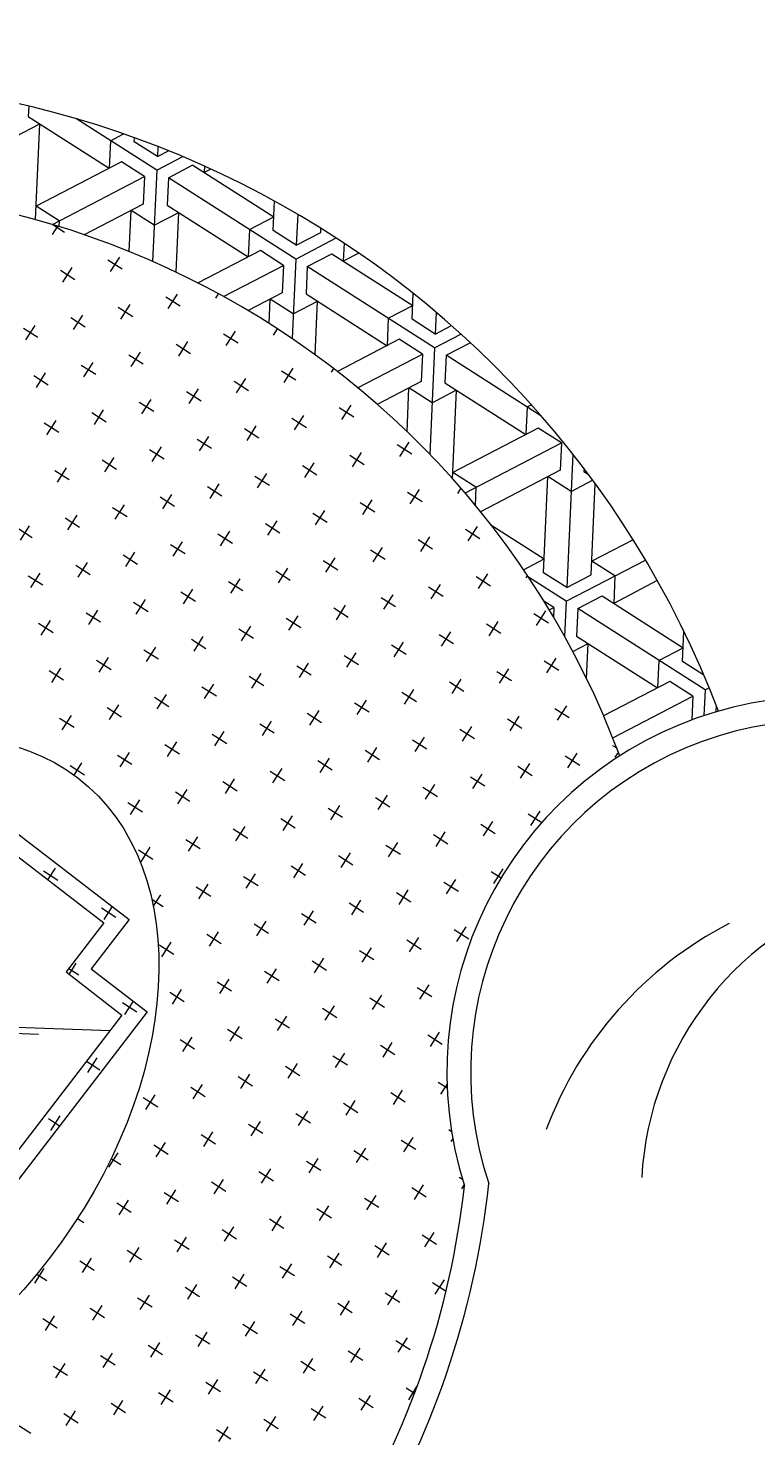
# Model space of a CAD drawing. Units: inches. Extents: x -4843 to -3402, y -164 to 3629.
# Tile 13 of 22: x -4487 to -4467, y 864 to 902. Entities that reach past the tile are written whole.
import ezdxf

# ---------------------------------------------------------------- set-up
doc = ezdxf.new("R2010")
doc.units = ezdxf.units.IN
doc.layers.add('A-ANNO-DIMS', color=2, linetype='Continuous', lineweight=18)
doc.layers.add('furniture', color=6, linetype='Continuous', lineweight=18)
doc.styles.get("Standard").update_dxf_attribs({"font": 'arial.ttf'})
doc.dimstyles.get("Standard").update_dxf_attribs({"dimtxt": 0.18, "dimasz": 0.18, "dimexe": 0.18, "dimexo": 0.0625, "dimgap": 0.09, "dimtad": 0, "dimtih": 1, "dimtoh": 1, "dimdec": 4, "dimzin": 0, "dimdsep": 46, "dimtxsty": 'Standard', "dimcen": 0.09, "dimadec": 0, "dimazin": 0, "dimtfac": 1, "dimtdec": 4, "dimtofl": 0, "dimtmove": 0, "dimatfit": 3, "dimfxl": 1, "dimtolj": 1, "dimtzin": 0, "dimarcsym": 0})

# ---------------------------------------------------------------- blocks, each defined once
blk = doc.blocks.new('A$C30AE1D3B')
for p, q in [((999.1, 1767.5, -685.7), (983.6, 1760.2, -685.7)), ((994.5, 1754.8, -685.7), (989.7, 1764.9, -685.7)), ((1049.7, 1749, -685.7), (1032.4, 1741, -685.7)), ((1045.1, 1736.4, -685.7), (1037, 1753.6, -685.7)), ((1095.7, 1717.9, -685.7), (1087.7, 1735.2, -685.7)), ((976, 1704.2, -685.7), (968, 1721.4, -685.7)), ((1100.3, 1730.6, -685.7), (1083.1, 1722.6, -685.7)), ((980.6, 1716.8, -685.7), (963.4, 1708.8, -685.7)), ((1026.7, 1685.7, -685.7), (1018.6, 1703, -685.7)), ((1151, 1712.2, -685.7), (1133.7, 1704.1, -685.7)), ((1146.3, 1699.5, -685.7), (1138.3, 1716.8, -685.7)), ((907, 1672, -685.7), (899.5, 1688, -685.7)), ((1031.3, 1698.4, -685.7), (1014, 1690.4, -685.7)), ((1201.6, 1693.7, -685.7), (1184.3, 1685.7, -685.7)), ((1197, 1681.1, -685.7), (1188.9, 1698.4, -685.7)), ((911.6, 1684.6, -685.7), (894.3, 1676.6, -685.7)), ((957.6, 1653.5, -685.7), (949.5, 1670.8, -685.7)), ((1081.9, 1680, -685.7), (1064.6, 1671.9, -685.7)), ((1077.3, 1667.3, -685.7), (1069.2, 1684.6, -685.7)), ((962.2, 1666.2, -685.7), (944.9, 1658.1, -685.7)), ((1132.5, 1661.5, -685.7), (1115.3, 1653.5, -685.7)), ((1127.9, 1648.9, -685.7), (1119.9, 1666.2, -685.7)), ((1012.8, 1647.8, -685.7), (995.6, 1639.7, -685.7)), ((1008.2, 1635.1, -685.7), (1000.2, 1652.4, -685.7)), ((1183.2, 1643.1, -685.7), (1165.9, 1635.1, -685.7)), ((1178.6, 1630.5, -685.7), (1170.5, 1647.7, -685.7)), ((893.1, 1634, -685.7), (875.9, 1625.9, -685.7)), ((888.5, 1621.3, -685.7), (880.5, 1638.6, -685.7)), ((1063.5, 1629.3, -685.7), (1046.2, 1621.3, -685.7)), ((1058.9, 1616.7, -685.7), (1050.8, 1633.9, -685.7)), ((1233.8, 1624.7, -685.7), (1216.5, 1616.6, -685.7)), ((1229.2, 1612, -685.7), (1221.1, 1629.3, -685.7)), ((943.8, 1615.6, -685.7), (926.5, 1607.5, -685.7)), ((939.2, 1602.9, -685.7), (931.1, 1620.2, -685.7)), ((1114.1, 1610.9, -685.7), (1096.8, 1602.9, -685.7)), ((1109.5, 1598.3, -685.7), (1101.4, 1615.5, -685.7)), ((1279.8, 1593.6, -685.7), (1271.8, 1610.9, -685.7)), ((819.5, 1589.1, -685.7), (817.6, 1593.1, -685.7)), ((824.1, 1601.8, -685.7), (819.4, 1599.6, -685.7)), ((994.4, 1597.1, -685.7), (977.1, 1589.1, -685.7)), ((989.8, 1584.5, -685.7), (981.7, 1601.7, -685.7)), ((1160.1, 1579.8, -685.7), (1152.1, 1597.1, -685.7)), ((1284.4, 1606.3, -685.7), (1267.2, 1598.2, -685.7)), ((874.7, 1583.4, -685.7), (857.4, 1575.3, -685.7)), ((870.1, 1570.7, -685.7), (862.1, 1588, -685.7)), ((1045, 1578.7, -685.7), (1027.8, 1570.7, -685.7)), ((1040.4, 1566.1, -685.7), (1032.4, 1583.3, -685.7)), ((1164.7, 1592.5, -685.7), (1147.5, 1584.4, -685.7)), ((1210.8, 1561.4, -685.7), (1202.7, 1578.7, -685.7)), ((1335.1, 1587.8, -685.7), (1317.8, 1579.8, -685.7)), ((1330.4, 1575.2, -685.7), (1322.4, 1592.4, -685.7)), ((925.3, 1564.9, -685.7), (908.1, 1556.9, -685.7)), ((920.7, 1552.3, -685.7), (912.7, 1569.5, -685.7)), ((1091.1, 1547.6, -685.7), (1083, 1564.9, -685.7)), ((1215.4, 1574.1, -685.7), (1198.1, 1566, -685.7)), ((1381.1, 1556.7, -685.7), (1373, 1574, -685.7)), ((805.7, 1551.2, -685.7), (802.7, 1549.8, -685.7)), ((976, 1546.5, -685.7), (958.7, 1538.5, -685.7)), ((971.4, 1533.8, -685.7), (963.3, 1551.1, -685.7)), ((1095.7, 1560.3, -685.7), (1078.4, 1552.2, -685.7)), ((1141.7, 1529.2, -685.7), (1133.6, 1546.5, -685.7)), ((1266, 1555.6, -685.7), (1248.7, 1547.6, -685.7)), ((1261.4, 1543, -685.7), (1253.3, 1560.2, -685.7)), ((801, 1538.5, -685.7), (799.4, 1542, -685.7)), ((856.3, 1532.7, -685.7), (839, 1524.7, -685.7)), ((851.7, 1520.1, -685.7), (843.6, 1537.3, -685.7)), ((1022, 1515.4, -685.7), (1014, 1532.7, -685.7)), ((1146.3, 1541.9, -685.7), (1129, 1533.8, -685.7)), ((1316.6, 1537.2, -685.7), (1299.4, 1529.1, -685.7)), ((1312, 1524.5, -685.7), (1304, 1541.8, -685.7)), ((902.3, 1501.6, -685.7), (894.3, 1518.9, -685.7)), ((1026.6, 1528.1, -685.7), (1009.3, 1520, -685.7)), ((1196.9, 1523.4, -685.7), (1179.7, 1515.4, -685.7)), ((1192.3, 1510.8, -685.7), (1184.3, 1528, -685.7)), ((787.2, 1500.5, -685.7), (775.6, 1495.1, -685.7)), ((906.9, 1514.3, -685.7), (889.7, 1506.3, -685.7)), ((952.9, 1483.2, -685.7), (944.9, 1500.5, -685.7)), ((1077.2, 1509.6, -685.7), (1060, 1501.6, -685.7)), ((1072.6, 1497, -685.7), (1064.6, 1514.3, -685.7)), ((1247.6, 1505, -685.7), (1230.3, 1496.9, -685.7)), ((1243, 1492.3, -685.7), (1234.9, 1509.6, -685.7)), ((782.6, 1487.9, -685.7), (777.6, 1498.6, -685.7)), ((833.2, 1469.4, -685.7), (825.2, 1486.7, -685.7)), ((957.5, 1495.9, -685.7), (940.3, 1487.8, -685.7)), ((1127.9, 1491.2, -685.7), (1110.6, 1483.2, -685.7)), ((1123.3, 1478.6, -685.7), (1115.2, 1495.8, -685.7)), ((1298.2, 1486.6, -685.7), (1280.9, 1478.5, -685.7)), ((1293.6, 1473.9, -685.7), (1285.5, 1491.2, -685.7)), ((837.9, 1482.1, -685.7), (820.6, 1474, -685.7)), ((883.9, 1451, -685.7), (875.8, 1468.3, -685.7)), ((1008.2, 1477.4, -685.7), (990.9, 1469.4, -685.7)), ((1003.6, 1464.8, -685.7), (995.5, 1482.1, -685.7)), ((1178.5, 1472.8, -685.7), (1161.2, 1464.7, -685.7)), ((1173.9, 1460.1, -685.7), (1165.8, 1477.4, -685.7)), ((764.2, 1437.2, -685.7), (756.1, 1454.5, -685.7)), ((888.5, 1463.7, -685.7), (871.2, 1455.6, -685.7)), ((1058.8, 1459, -685.7), (1041.5, 1451, -685.7)), ((1054.2, 1446.4, -685.7), (1046.2, 1463.6, -685.7)), ((1229.1, 1454.4, -685.7), (1211.9, 1446.3, -685.7)), ((1224.5, 1441.7, -685.7), (1216.5, 1459, -685.7)), ((768.8, 1449.9, -685.7), (751.5, 1441.8, -685.7)), ((939.1, 1445.2, -685.7), (921.9, 1437.2, -685.7)), ((934.5, 1432.6, -685.7), (926.5, 1449.9, -685.7)), ((1013.2, 1248.8, -685.7), (1537, 1439.4, -685.7)), ((1109.4, 1440.6, -685.7), (1092.2, 1432.5, -685.7)), ((1104.8, 1427.9, -685.7), (1096.8, 1445.2, -685.7)), ((1272.7, 1428.6, -685.7), (1267.1, 1440.5, -685.7)), ((819.4, 1431.5, -685.7), (802.2, 1423.4, -685.7)), ((814.8, 1418.8, -685.7), (806.8, 1436.1, -685.7)), ((989.8, 1426.8, -685.7), (972.5, 1418.8, -685.7)), ((985.1, 1414.2, -685.7), (977.1, 1431.4, -685.7)), ((1160.1, 1422.2, -685.7), (1142.8, 1414.1, -685.7)), ((1155.5, 1409.5, -685.7), (1147.4, 1426.8, -685.7)), ((1279.8, 1435.9, -685.7), (1262.5, 1427.9, -685.7)), ((870.1, 1413, -685.7), (852.8, 1405, -685.7)), ((865.5, 1400.4, -685.7), (857.4, 1417.6, -685.7)), ((1040.4, 1408.4, -685.7), (1023.1, 1400.3, -685.7)), ((1035.8, 1395.7, -685.7), (1027.7, 1413, -685.7)), ((1038.9, 1236.8, -685.7), (1525.1, 1413.8, -685.7)), ((1201.6, 1400.8, -685.7), (1198.1, 1408.3, -685.7)), ((750.4, 1399.3, -685.7), (733.1, 1391.2, -685.7)), ((745.8, 1386.6, -685.7), (737.7, 1403.9, -685.7)), ((920.7, 1394.6, -685.7), (903.4, 1386.6, -685.7)), ((916.1, 1382, -685.7), (908, 1399.2, -685.7)), ((1091, 1390, -685.7), (1073.8, 1381.9, -685.7)), ((1086.4, 1377.3, -685.7), (1078.4, 1394.6, -685.7)), ((801, 1380.8, -685.7), (783.7, 1372.8, -685.7)), ((796.4, 1368.2, -685.7), (788.3, 1385.4, -685.7)), ((971.3, 1376.2, -685.7), (954.1, 1368.1, -685.7)), ((966.7, 1363.5, -685.7), (958.7, 1380.8, -685.7)), ((1134.3, 1364.7, -685.7), (1129, 1376.1, -685.7)), ((681.3, 1367.1, -685.7), (664, 1359, -685.7)), ((676.7, 1354.4, -685.7), (668.6, 1371.7, -685.7)), ((851.6, 1362.4, -685.7), (834.4, 1354.4, -685.7)), ((847, 1349.7, -685.7), (839, 1367, -685.7)), ((1017.3, 1345.1, -685.7), (1009.3, 1362.4, -685.7)), ((1141.6, 1371.5, -685.7), (1124.4, 1363.5, -685.7)), ((731.9, 1348.6, -685.7), (714.7, 1340.6, -685.7)), ((727.3, 1336, -685.7), (719.3, 1353.2, -685.7)), ((902.3, 1344, -685.7), (885, 1335.9, -685.7)), ((897.7, 1331.3, -685.7), (889.6, 1348.6, -685.7)), ((1022, 1357.8, -685.7), (1004.7, 1349.7, -685.7)), ((1068, 1326.7, -685.7), (1059.9, 1343.9, -685.7)), ((612.2, 1334.9, -685.7), (595, 1326.8, -685.7)), ((607.6, 1322.2, -685.7), (602.2, 1333.9, -685.7)), ((782.6, 1330.2, -685.7), (765.3, 1322.2, -685.7)), ((778, 1317.5, -685.7), (769.9, 1334.8, -685.7)), ((948.3, 1312.9, -685.7), (940.2, 1330.2, -685.7)), ((1072.6, 1339.3, -685.7), (1055.3, 1331.3, -685.7)), ((662.9, 1316.4, -685.7), (645.6, 1308.4, -685.7)), ((658.3, 1303.8, -685.7), (650.2, 1321, -685.7)), ((833.2, 1311.8, -685.7), (815.9, 1303.7, -685.7)), ((828.6, 1299.1, -685.7), (820.5, 1316.4, -685.7)), ((952.9, 1325.6, -685.7), (935.6, 1317.5, -685.7)), ((998.9, 1294.5, -685.7), (990.9, 1311.7, -685.7)), ((298.1, 1300.5, -685.7), (302.2, 1306.3, -685.7)), ((299.5, 1279.4, -685.7), (315.8, 1302.7, -685.7)), ((314.6, 1278, -685.7), (329.7, 1299.5, -685.7)), ((543.2, 1302.7, -685.7), (525.9, 1294.6, -685.7)), ((538.6, 1290, -685.7), (531, 1306.3, -685.7)), ((713.5, 1298, -685.7), (696.2, 1289.9, -685.7)), ((708.9, 1285.3, -685.7), (700.9, 1302.6, -685.7)), ((879.2, 1280.7, -685.7), (871.2, 1298, -685.7)), ((1003.5, 1307.1, -685.7), (986.3, 1299.1, -685.7)), ((1173.9, 1302.5, -685.7), (1156.6, 1294.4, -685.7)), ((1169.2, 1289.8, -685.7), (1163, 1303.3, -685.7)), ((418.9, 1276.2, -685.7), (416.6, 1281.1, -685.7)), ((423.5, 1288.9, -685.7), (417.7, 1286.2, -685.7)), ((593.8, 1284.2, -685.7), (576.6, 1276.2, -685.7)), ((589.2, 1271.6, -685.7), (581.2, 1288.8, -685.7)), ((759.5, 1266.9, -685.7), (751.5, 1284.2, -685.7)), ((883.8, 1293.3, -685.7), (866.6, 1285.3, -685.7)), ((1041.5, 1293.2, -685.7), (1041.5, 1293.3, -685.7)), ((299.4, 1279.4, -685.7), (294.3, 1279.8, -685.7)), ((299.4, 1279.4, -685.7), (370.3, 1127.4, -685.7)), ((314.6, 1278, -685.7), (327.5, 1250.4, -685.7)), ((414.3, 1269.3, -685.7), (314.6, 1278, -685.7)), ((474.1, 1270.5, -685.7), (456.9, 1262.4, -685.7)), ((469.5, 1257.8, -685.7), (461.5, 1275.1, -685.7)), ((644.4, 1265.8, -685.7), (627.2, 1257.7, -685.7)), ((639.8, 1253.1, -685.7), (631.8, 1270.4, -685.7)), ((764.1, 1279.6, -685.7), (746.9, 1271.5, -685.7)), ((810.2, 1248.5, -685.7), (802.1, 1265.8, -685.7)), ((934.5, 1274.9, -685.7), (917.2, 1266.9, -685.7)), ((929.9, 1262.3, -685.7), (921.8, 1279.5, -685.7)), ((1104.8, 1270.3, -685.7), (1087.5, 1262.2, -685.7)), ((1099.6, 1258.9, -685.7), (1092.1, 1274.9, -685.7)), ((291.7, 1264.8, -685.7), (303.6, 1239.3, -685.7)), ((327.5, 1250.4, -685.7), (409.8, 1243.2, -685.7)), ((524.8, 1252, -685.7), (507.5, 1244, -685.7)), ((520.1, 1239.4, -685.7), (512.1, 1256.6, -685.7)), ((690.5, 1234.7, -685.7), (682.4, 1252, -685.7)), ((814.8, 1261.1, -685.7), (797.5, 1253.1, -685.7)), ((985.1, 1256.5, -685.7), (967.8, 1248.4, -685.7)), ((980.5, 1243.8, -685.7), (972.4, 1261.1, -685.7)), ((303.6, 1239.3, -685.7), (284.4, 1211.8, -685.7)), ((325.2, 1224.1, -685.7), (342.7, 1249.1, -685.7)), ((387.8, 1152.4, -685.7), (342.7, 1249.1, -685.7)), ((575.4, 1233.6, -685.7), (558.1, 1225.5, -685.7)), ((570.8, 1220.9, -685.7), (562.7, 1238.2, -685.7)), ((695.1, 1247.4, -685.7), (677.8, 1239.3, -685.7)), ((865.4, 1242.7, -685.7), (848.1, 1234.7, -685.7)), ((860.8, 1230.1, -685.7), (852.7, 1247.3, -685.7)), ((1040, 1175.2, -685.7), (1013.2, 1248.8, -685.7)), ((1035.7, 1238.1, -685.7), (1019.8, 1230.6, -685.7)), ((1031.1, 1225.4, -685.7), (1023.1, 1242.7, -685.7)), ((1065.6, 1163.2, -685.7), (1038.9, 1236.8, -685.7)), ((1381.8, 1022.6, -685.7), (1059.1, 1244.3, -685.7)), ((339.9, 1130.1, -685.7), (294.8, 1226.8, -685.7)), ((325.2, 1224.1, -685.7), (294.8, 1226.8, -685.7)), ((455.7, 1219.8, -685.7), (438.4, 1211.8, -685.7)), ((451.1, 1207.2, -685.7), (443, 1224.4, -685.7)), ((621.4, 1202.5, -685.7), (613.4, 1219.8, -685.7)), ((745.7, 1228.9, -685.7), (728.4, 1220.9, -685.7)), ((741.1, 1216.3, -685.7), (733.1, 1233.5, -685.7)), ((916, 1224.3, -685.7), (898.8, 1216.2, -685.7)), ((911.4, 1211.6, -685.7), (903.4, 1228.9, -685.7)), ((501.7, 1188.7, -685.7), (493.7, 1206, -685.7)), ((626, 1215.2, -685.7), (608.8, 1207.1, -685.7)), ((796.3, 1210.5, -685.7), (779.1, 1202.5, -685.7)), ((791.7, 1197.9, -685.7), (783.7, 1215.1, -685.7)), ((966.7, 1205.9, -685.7), (949.4, 1197.8, -685.7)), ((962.1, 1193.2, -685.7), (954, 1210.5, -685.7)), ((1451, 983.2, -685.7), (1128.3, 1204.9, -685.7)), ((403.6, 1198, -685.7), (381.3, 1166.2, -685.7)), ((506.3, 1201.4, -685.7), (489.1, 1193.3, -685.7)), ((552.4, 1170.3, -685.7), (544.3, 1187.6, -685.7)), ((676.7, 1196.7, -685.7), (659.4, 1188.7, -685.7)), ((672, 1184.1, -685.7), (664, 1201.3, -685.7)), ((847, 1192.1, -685.7), (829.7, 1184, -685.7)), ((842.4, 1179.4, -685.7), (834.3, 1196.7, -685.7)), ((432.7, 1156.5, -685.7), (424.6, 1173.8, -685.7)), ((557, 1183, -685.7), (539.7, 1174.9, -685.7)), ((727.3, 1178.3, -685.7), (710, 1170.3, -685.7)), ((722.7, 1165.6, -685.7), (714.6, 1182.9, -685.7)), ((897.6, 1173.7, -685.7), (880.3, 1165.6, -685.7)), ((893, 1161, -685.7), (885, 1178.3, -685.7)), ((975.3, 1151.6, -685.7), (1040, 1175.2, -685.7)), ((1060.9, 1161.5, -685.7), (1055.3, 1173.6, -685.7)), ((400.4, 1164.5, -685.7), (381.3, 1166.2, -685.7)), ((437.3, 1169.2, -685.7), (420, 1161.1, -685.7)), ((607.6, 1164.5, -685.7), (590.3, 1156.5, -685.7)), ((603, 1151.9, -685.7), (594.9, 1169.1, -685.7)), ((777.9, 1159.9, -685.7), (760.7, 1151.8, -685.7)), ((773.3, 1147.2, -685.7), (765.3, 1164.5, -685.7)), ((942, 1146, -685.7), (935.6, 1159.8, -685.7)), ((1001, 1139.7, -685.7), (1065.6, 1163.2, -685.7)), ((1064.2, 1167.2, -685.7), (1050.7, 1160.9, -685.7)), ((279.1, 1148.6, -685.7), (333.5, 1143.9, -685.7)), ((316, 1118.9, -685.7), (333.5, 1143.9, -685.7)), ((370.3, 1127.4, -685.7), (387.8, 1152.4, -685.7)), ((376.7, 1113.6, -685.7), (399.1, 1145.6, -685.7)), ((487.9, 1150.8, -685.7), (470.6, 1142.7, -685.7)), ((483.3, 1138.1, -685.7), (475.2, 1155.4, -685.7)), ((658.2, 1146.1, -685.7), (641, 1138.1, -685.7)), ((653.6, 1133.4, -685.7), (645.6, 1150.7, -685.7)), ((828.5, 1141.5, -685.7), (811.3, 1133.4, -685.7)), ((823.9, 1128.8, -685.7), (815.9, 1146.1, -685.7)), ((944.9, 1153.7, -685.7), (931, 1147.2, -685.7)), ((1075.8, 875.5, -685.7), (975.3, 1151.6, -685.7)), ((994.3, 1124.1, -685.7), (986.2, 1141.4, -685.7)), ((370.3, 1127.4, -685.7), (339.9, 1130.1, -685.7)), ((538.5, 1132.3, -685.7), (521.3, 1124.3, -685.7)), ((533.9, 1119.7, -685.7), (525.9, 1136.9, -685.7)), ((708.9, 1127.7, -685.7), (691.6, 1119.6, -685.7)), ((704.2, 1115, -685.7), (696.2, 1132.3, -685.7)), ((874.6, 1110.4, -685.7), (866.5, 1127.6, -685.7)), ((998.9, 1136.8, -685.7), (983.4, 1129.6, -685.7)), ((1087.8, 901.2, -685.7), (1001, 1139.7, -685.7)), ((376.7, 1113.6, -685.7), (278, 1122.3, -685.7)), ((316, 1118.9, -685.7), (328.9, 1091.3, -685.7)), ((376.7, 1113.6, -685.7), (397.7, 1068.6, -685.7)), ((391.9, 1112.3, -685.7), (398, 1121, -685.7)), ((391.9, 1112.3, -685.7), (397.5, 1100.2, -685.7)), ((397.7, 1111.8, -685.7), (391.9, 1112.3, -685.7)), ((418.8, 1118.6, -685.7), (401.6, 1110.5, -685.7)), ((414.2, 1105.9, -685.7), (406.2, 1123.2, -685.7)), ((589.2, 1113.9, -685.7), (571.9, 1105.8, -685.7)), ((584.6, 1101.2, -685.7), (576.5, 1118.5, -685.7)), ((759.5, 1109.2, -685.7), (742.2, 1101.2, -685.7)), ((754.9, 1096.6, -685.7), (746.8, 1113.9, -685.7)), ((879.2, 1123, -685.7), (861.9, 1115, -685.7)), ((925.2, 1091.9, -685.7), (917.2, 1109.2, -685.7)), ((277.5, 1095.8, -685.7), (328.9, 1091.3, -685.7)), ((337.6, 1103.8, -685.7), (279.6, 1021, -685.7)), ((283, 979.8, -685.7), (368, 1101.1, -685.7)), ((368, 1101.1, -685.7), (337.6, 1103.8, -685.7)), ((368, 1101.1, -685.7), (380.9, 1073.5, -685.7)), ((469.5, 1100.1, -685.7), (452.2, 1092.1, -685.7)), ((464.9, 1087.5, -685.7), (456.8, 1104.7, -685.7)), ((639.8, 1095.5, -685.7), (622.5, 1087.4, -685.7)), ((635.2, 1082.8, -685.7), (627.1, 1100.1, -685.7)), ((805.5, 1078.2, -685.7), (797.5, 1095.4, -685.7)), ((929.8, 1104.6, -685.7), (912.5, 1096.5, -685.7)), ((520.1, 1081.7, -685.7), (502.8, 1073.6, -685.7)), ((515.5, 1069, -685.7), (507.4, 1086.3, -685.7)), ((685.8, 1064.4, -685.7), (677.8, 1081.7, -685.7)), ((810.1, 1090.8, -685.7), (792.9, 1082.8, -685.7)), ((380.9, 1073.5, -685.7), (319.7, 986.1, -685.7)), ((400.4, 1067.9, -685.7), (397.7, 1066.7, -685.7)), ((570.7, 1063.3, -685.7), (553.5, 1055.2, -685.7)), ((566.1, 1050.6, -685.7), (558.1, 1067.9, -685.7)), ((690.4, 1077, -685.7), (673.2, 1069, -685.7)), ((736.5, 1046, -685.7), (728.4, 1063.2, -685.7)), ((860.8, 1072.4, -685.7), (843.5, 1064.3, -685.7)), ((856.1, 1059.7, -685.7), (848.1, 1077, -685.7)), ((1027.7, 1066.2, -685.7), (1013.8, 1059.7, -685.7)), ((1026.5, 1055.1, -685.7), (1018.4, 1072.3, -685.7)), ((401.9, 997.2, -685.7), (372.1, 1061, -685.7)), ((398, 1058.8, -685.7), (372.1, 1061, -685.7)), ((451, 1049.5, -685.7), (433.8, 1041.4, -685.7)), ((446.4, 1036.8, -685.7), (438.4, 1054.1, -685.7)), ((616.8, 1032.2, -685.7), (608.7, 1049.4, -685.7)), ((741.1, 1058.6, -685.7), (723.8, 1050.6, -685.7)), ((911.4, 1054, -685.7), (894.1, 1045.9, -685.7)), ((906.8, 1041.3, -685.7), (898.7, 1058.6, -685.7)), ((501.7, 1031.1, -685.7), (484.4, 1023, -685.7)), ((497.1, 1018.4, -685.7), (489, 1035.7, -685.7)), ((621.4, 1044.8, -685.7), (604.1, 1036.8, -685.7)), ((667.4, 1013.8, -685.7), (659.3, 1031, -685.7)), ((791.7, 1040.2, -685.7), (774.4, 1032.1, -685.7)), ((787.1, 1027.5, -685.7), (779, 1044.8, -685.7)), ((306.8, 1013.7, -685.7), (280, 1016.1, -685.7)), ((547.7, 1000, -685.7), (539.6, 1017.2, -685.7)), ((672, 1026.4, -685.7), (654.7, 1018.4, -685.7)), ((842.3, 1021.8, -685.7), (825.1, 1013.7, -685.7)), ((837.7, 1009.1, -685.7), (829.7, 1026.4, -685.7)), ((282.9, 1002.6, -685.7), (280.6, 1007.6, -685.7)), ((281.1, 1000.1, -685.7), (282.9, 1002.6, -685.7)), ((306.8, 1013.8, -685.7), (319.7, 986.1, -685.7)), ((428, 986.2, -685.7), (420, 1003.5, -685.7)), ((552.3, 1012.6, -685.7), (535, 1004.6, -685.7)), ((722.6, 1008, -685.7), (705.4, 999.9, -685.7)), ((718, 995.3, -685.7), (710, 1012.6, -685.7)), ((893, 1003.3, -685.7), (875.7, 995.3, -685.7)), ((888.3, 990.7, -685.7), (880.3, 1007.9, -685.7)), ((287, 962.5, -685.7), (304.5, 987.5, -685.7)), ((304.5, 987.4, -685.7), (403.8, 978.8, -685.7)), ((432.6, 998.9, -685.7), (415.3, 990.8, -685.7)), ((478.6, 967.8, -685.7), (470.6, 985, -685.7)), ((602.9, 994.2, -685.7), (585.7, 986.2, -685.7)), ((598.3, 981.5, -685.7), (590.3, 998.8, -685.7)), ((773.3, 989.6, -685.7), (756, 981.5, -685.7)), ((768.7, 976.9, -685.7), (760.6, 994.2, -685.7)), ((939, 972.2, -685.7), (930.9, 989.5, -685.7)), ((393.3, 953.2, -685.7), (404.9, 969.7, -685.7)), ((483.2, 980.4, -685.7), (466, 972.4, -685.7)), ((653.6, 975.8, -685.7), (636.3, 967.7, -685.7)), ((649, 963.1, -685.7), (640.9, 980.4, -685.7)), ((823.9, 971.1, -685.7), (806.6, 963.1, -685.7)), ((819.3, 958.5, -685.7), (811.2, 975.7, -685.7)), ((940.9, 983.6, -685.7), (926.3, 976.8, -685.7)), ((287, 962.5, -685.7), (299.9, 934.9, -685.7)), ((407.3, 952, -685.7), (287, 962.5, -685.7)), ((393.3, 953.2, -685.7), (406.2, 925.6, -685.7)), ((533.9, 962, -685.7), (516.6, 954, -685.7)), ((529.3, 949.3, -685.7), (521.2, 966.6, -685.7)), ((704.2, 957.4, -685.7), (686.9, 949.3, -685.7)), ((699.6, 944.7, -685.7), (691.5, 962, -685.7)), ((874.5, 952.7, -685.7), (857.3, 944.6, -685.7)), ((869.9, 940, -685.7), (861.9, 957.3, -685.7)), ((414.2, 948.2, -685.7), (408.2, 945.5, -685.7)), ((584.5, 943.6, -685.7), (567.2, 935.5, -685.7)), ((579.9, 930.9, -685.7), (571.9, 948.2, -685.7)), ((754.8, 938.9, -685.7), (737.6, 930.9, -685.7)), ((750.2, 926.3, -685.7), (742.2, 943.5, -685.7)), ((920.6, 921.6, -685.7), (912.5, 938.9, -685.7)), ((290, 924.9, -685.7), (342.7, 811.9, -685.7)), ((297.6, 908.6, -685.7), (315.1, 933.5, -685.7)), ((299.9, 934.9, -685.7), (406.2, 925.6, -685.7)), ((360.2, 836.9, -685.7), (315.1, 933.5, -685.7)), ((410.4, 931.6, -685.7), (353.7, 850.7, -685.7)), ((464.8, 929.8, -685.7), (447.6, 921.7, -685.7)), ((460.2, 917.1, -685.7), (452.2, 934.4, -685.7)), ((635.1, 925.1, -685.7), (617.9, 917.1, -685.7)), ((630.5, 912.5, -685.7), (622.5, 929.8, -685.7)), ((800.9, 907.8, -685.7), (792.8, 925.1, -685.7)), ((925.2, 934.3, -685.7), (907.9, 926.2, -685.7)), ((297.6, 908.6, -685.7), (292.5, 909, -685.7)), ((515.4, 911.4, -685.7), (498.2, 903.3, -685.7)), ((510.8, 898.7, -685.7), (502.8, 916, -685.7)), ((685.8, 906.7, -685.7), (668.5, 898.7, -685.7)), ((681.2, 894.1, -685.7), (673.1, 911.3, -685.7)), ((805.5, 920.5, -685.7), (788.2, 912.4, -685.7)), ((851.5, 889.4, -685.7), (843.4, 906.7, -685.7)), ((349.1, 798.1, -685.7), (417.1, 895.2, -685.7)), ((566.1, 892.9, -685.7), (548.8, 884.9, -685.7)), ((561.5, 880.3, -685.7), (553.4, 897.6, -685.7)), ((731.8, 875.6, -685.7), (723.7, 892.9, -685.7)), ((856.1, 902.1, -685.7), (838.8, 894, -685.7)), ((446.4, 879.2, -685.7), (429.1, 871.1, -685.7)), ((441.8, 866.5, -685.7), (433.7, 883.8, -685.7)), ((616.7, 874.5, -685.7), (599.4, 866.5, -685.7)), ((612.1, 861.9, -685.7), (604.1, 879.1, -685.7)), ((736.4, 888.3, -685.7), (719.1, 880.2, -685.7)), ((782.4, 857.2, -685.7), (774.4, 874.5, -685.7)), ((906.7, 883.6, -685.7), (889.5, 875.6, -685.7)), ((902.1, 871, -685.7), (894.1, 888.2, -685.7)), ((424.9, 860.3, -685.7), (397, 820.4, -685.7)), ((497, 860.7, -685.7), (479.8, 852.7, -685.7)), ((492.4, 848.1, -685.7), (484.4, 865.3, -685.7)), ((662.7, 843.4, -685.7), (654.7, 860.7, -685.7)), ((787, 869.9, -685.7), (769.8, 861.8, -685.7)), ((384.1, 848, -685.7), (353.7, 850.6, -685.7)), ((384.1, 848, -685.7), (397, 820.4, -685.7)), ((543, 829.7, -685.7), (535, 846.9, -685.7)), ((667.3, 856.1, -685.7), (650.1, 848, -685.7)), ((837.7, 851.4, -685.7), (820.4, 843.4, -685.7)), ((833.1, 838.8, -685.7), (825, 856, -685.7)), ((342.7, 811.9, -685.7), (360.2, 836.9, -685.7)), ((547.7, 842.3, -685.7), (530.4, 834.3, -685.7)), ((593.7, 811.2, -685.7), (585.6, 828.5, -685.7)), ((718, 837.7, -685.7), (700.7, 829.6, -685.7)), ((713.4, 825, -685.7), (705.3, 842.3, -685.7)), ((888.3, 833, -685.7), (871, 825, -685.7)), ((883.7, 820.3, -685.7), (875.6, 837.6, -685.7)), ((342.7, 811.9, -685.7), (312.7, 814.5, -685.7)), ((364.3, 796.7, -685.7), (381.8, 821.7, -685.7)), ((381.8, 821.7, -685.7), (436.6, 816.9, -685.7)), ((474, 797.4, -685.7), (465.9, 814.7, -685.7)), ((598.3, 823.9, -685.7), (581, 815.8, -685.7)), ((768.6, 819.2, -685.7), (751.3, 811.2, -685.7)), ((764, 806.6, -685.7), (756, 823.8, -685.7)), ((349.1, 798.1, -685.7), (316.4, 800.9, -685.7)), ((349.1, 798.1, -685.7), (420, 646.1, -685.7)), ((364.3, 796.7, -685.7), (377.2, 769.1, -685.7)), ((445, 789.7, -685.7), (364.3, 796.7, -685.7)), ((478.6, 810.1, -685.7), (461.3, 802.1, -685.7)), ((648.9, 805.5, -685.7), (631.7, 797.4, -685.7)), ((644.3, 792.8, -685.7), (636.3, 810.1, -685.7)), ((819.2, 800.8, -685.7), (802, 792.7, -685.7)), ((814.6, 788.1, -685.7), (806.6, 805.4, -685.7)), ((340.4, 785.6, -685.7), (320.2, 787.3, -685.7)), ((326.6, 765.9, -685.7), (340.4, 785.6, -685.7)), ((340.4, 785.6, -685.7), (353.3, 758, -685.7)), ((529.2, 791.7, -685.7), (512, 783.6, -685.7)), ((524.6, 779, -685.7), (516.6, 796.3, -685.7)), ((699.5, 787, -685.7), (682.3, 779, -685.7)), ((694.9, 774.4, -685.7), (686.9, 791.6, -685.7)), ((869.9, 782.4, -685.7), (852.6, 774.3, -685.7)), ((865.3, 769.7, -685.7), (857.2, 787, -685.7)), ((374.9, 742.8, -685.7), (392.4, 767.8, -685.7)), ((377.2, 769.1, -685.7), (454.3, 762.4, -685.7)), ((437.4, 671.1, -685.7), (392.4, 767.8, -685.7)), ((579.9, 773.3, -685.7), (562.6, 765.2, -685.7)), ((575.2, 760.6, -685.7), (567.2, 777.9, -685.7)), ((750.2, 768.6, -685.7), (732.9, 760.5, -685.7)), ((745.6, 755.9, -685.7), (737.5, 773.2, -685.7)), ((353.3, 758, -685.7), (336.9, 734.6, -685.7)), ((460.2, 759.5, -685.7), (456, 757.6, -685.7)), ((630.5, 754.8, -685.7), (613.2, 746.8, -685.7)), ((625.9, 742.2, -685.7), (617.8, 759.4, -685.7)), ((800.8, 750.2, -685.7), (783.5, 742.1, -685.7)), ((796.2, 737.5, -685.7), (788.2, 754.8, -685.7)), ((389.6, 648.8, -685.7), (344.5, 745.5, -685.7)), ((374.9, 742.8, -685.7), (344.5, 745.5, -685.7)), ((510.8, 741, -685.7), (493.5, 733, -685.7)), ((506.2, 728.4, -685.7), (498.1, 745.7, -685.7)), ((681.1, 736.4, -685.7), (663.9, 728.3, -685.7)), ((676.5, 723.7, -685.7), (668.5, 741, -685.7)), ((846.8, 719.1, -685.7), (838.8, 736.3, -685.7)), ((465.1, 733.6, -685.7), (431, 684.9, -685.7)), ((561.4, 722.6, -685.7), (544.2, 714.6, -685.7)), ((556.8, 710, -685.7), (548.8, 727.2, -685.7)), ((727.1, 705.3, -685.7), (719.1, 722.6, -685.7)), ((851.4, 731.7, -685.7), (834.2, 723.7, -685.7)), ((426.4, 632.3, -685.7), (477.1, 704.7, -685.7)), ((612.1, 704.2, -685.7), (594.8, 696.1, -685.7)), ((607.5, 691.5, -685.7), (599.4, 708.8, -685.7)), ((731.8, 718, -685.7), (714.5, 709.9, -685.7)), ((777.8, 686.9, -685.7), (769.7, 704.1, -685.7)), ((492.4, 690.4, -685.7), (485, 687, -685.7)), ((658.1, 673.1, -685.7), (650, 690.4, -685.7)), ((782.4, 699.5, -685.7), (765.1, 691.5, -685.7)), ((461.4, 682.2, -685.7), (431, 684.9, -685.7)), ((461.4, 682.3, -685.7), (474.3, 654.6, -685.7)), ((489.7, 676.7, -685.7), (474.3, 654.6, -685.7)), ((543, 672, -685.7), (525.7, 663.9, -685.7)), ((538.4, 659.3, -685.7), (530.3, 676.6, -685.7)), ((662.7, 685.8, -685.7), (645.4, 677.7, -685.7)), ((708.7, 654.7, -685.7), (700.7, 671.9, -685.7)), ((363.8, 664.3, -685.7), (383.2, 662.6, -685.7)), ((371.7, 646.2, -685.7), (383.2, 662.6, -685.7)), ((420, 646.1, -685.7), (437.5, 671.1, -685.7)), ((441.6, 631, -685.7), (459.1, 656, -685.7)), ((459.1, 656, -685.7), (501.6, 652.2, -685.7)), ((589, 640.9, -685.7), (581, 658.2, -685.7)), ((713.3, 667.3, -685.7), (696.1, 659.3, -685.7)), ((420, 646.1, -685.7), (389.6, 648.8, -685.7)), ((593.6, 653.6, -685.7), (576.4, 645.5, -685.7)), ((764, 648.9, -685.7), (746.7, 640.9, -685.7)), ((759.3, 636.2, -685.7), (751.3, 653.5, -685.7)), ((426.4, 632.3, -685.7), (376, 636.7, -685.7)), ((426.4, 632.3, -685.7), (497.3, 480.4, -685.7)), ((441.6, 631, -685.7), (454.5, 603.4, -685.7)), ((516.3, 624.5, -685.7), (441.6, 631, -685.7)), ((644.3, 635.1, -685.7), (627, 627.1, -685.7)), ((639.7, 622.5, -685.7), (631.6, 639.7, -685.7)), ((387.3, 622.5, -685.7), (384.5, 618.5, -685.7)), ((417.7, 619.8, -685.7), (387.3, 622.5, -685.7)), ((397.9, 591.6, -685.7), (417.7, 619.8, -685.7)), ((417.7, 619.8, -685.7), (430.5, 592.2, -685.7)), ((524.6, 621.4, -685.7), (519.3, 618.9, -685.7)), ((694.9, 616.7, -685.7), (677.6, 608.7, -685.7)), ((690.3, 604, -685.7), (682.2, 621.3, -685.7)), ((452.2, 577.1, -685.7), (469.7, 602, -685.7)), ((454.5, 603.4, -685.7), (532.1, 596.6, -685.7)), ((514.7, 505.4, -685.7), (469.7, 602.1, -685.7)), ((575.2, 602.9, -685.7), (557.9, 594.9, -685.7)), ((570.6, 590.3, -685.7), (562.5, 607.5, -685.7)), ((745.5, 598.3, -685.7), (728.3, 590.2, -685.7)), ((740.9, 585.6, -685.7), (732.9, 602.9, -685.7)), ((430.6, 592.2, -685.7), (411.8, 565.4, -685.7)), ((466.9, 483.1, -685.7), (421.8, 579.7, -685.7)), ((452.2, 577.1, -685.7), (421.8, 579.7, -685.7)), ((625.8, 584.5, -685.7), (608.6, 576.4, -685.7)), ((621.2, 571.8, -685.7), (613.2, 589.1, -685.7)), ((546.2, 573.3, -685.7), (508.3, 519.2, -685.7)), ((676.5, 566.1, -685.7), (659.2, 558, -685.7)), ((671.9, 553.4, -685.7), (663.8, 570.7, -685.7)), ((503.7, 466.6, -685.7), (561.8, 549.5, -685.7)), ((727.1, 547.6, -685.7), (709.8, 539.6, -685.7)), ((722.5, 535, -685.7), (714.4, 552.2, -685.7)), ((607.4, 533.9, -685.7), (590.1, 525.8, -685.7)), ((602.8, 521.2, -685.7), (594.7, 538.5, -685.7)), ((538.7, 516.5, -685.7), (508.3, 519.2, -685.7)), ((538.7, 516.5, -685.7), (551.5, 488.9, -685.7)), ((577.8, 526.3, -685.7), (551.6, 488.9, -685.7)), ((658, 515.4, -685.7), (640.8, 507.4, -685.7)), ((653.4, 502.8, -685.7), (645.4, 520, -685.7)), ((497.3, 480.4, -685.7), (514.8, 505.4, -685.7)), ((452.3, 497.6, -685.7), (460.5, 496.8, -685.7)), ((456.5, 491.1, -685.7), (460.5, 496.9, -685.7)), ((518.9, 465.3, -685.7), (536.4, 490.2, -685.7)), ((536.4, 490.2, -685.7), (609.9, 483.8, -685.7)), ((497.3, 480.4, -685.7), (466.9, 483, -685.7)), ((503.7, 466.6, -685.7), (471.1, 469.4, -685.7)), ((633.4, 455.5, -685.7), (627, 469.4, -685.7)), ((495, 454.1, -685.7), (481, 455.3, -685.7)), ((488.6, 444.9, -685.7), (495, 454.1, -685.7)), ((495, 454.1, -685.7), (507.8, 426.5, -685.7)), ((503.7, 466.6, -685.7), (548.7, 370.1, -685.7)), ((518.9, 465.3, -685.7), (531.8, 437.6, -685.7)), ((633.7, 455.2, -685.7), (518.9, 465.2, -685.7)), ((625.2, 456, -685.7), (628.7, 461, -685.7)), ((625.2, 456, -685.7), (638, 428.3, -685.7)), ((639.6, 464.8, -685.7), (629.5, 460.1, -685.7)), ((531.8, 437.6, -685.7), (638, 428.3, -685.7)), ((646.6, 440.6, -685.7), (585.6, 353.4, -685.7)), ((507.9, 426.5, -685.7), (505.3, 422.8, -685.7)), ((529.5, 411.3, -685.7), (547, 436.3, -685.7)), ((592, 339.6, -685.7), (546.9, 436.3, -685.7)), ((529.5, 411.3, -685.7), (513.1, 412.7, -685.7)), ((616, 350.8, -685.7), (585.6, 353.4, -685.7)), ((585.5, 330.3, -685.7), (592, 339.6, -685.7))]:
    blk.add_line(p, q)
for centre, radius, start, end in [((1588.1, -668.8, -685.7), 3092.5, 90.4124, 113.4876), ((1588.1, -668.8, -685.7), 3066.1, 90.5286, 113.4647), ((1564.8, 996.8, -685.7), 985.5, 91.1759, 141.3181), ((1550.3, 1015.2, -685.7), 936.1, 90.475, 141.314), ((416.7, 1707.2, -685.7), 416.9, 169.0069, 345.147), ((416.7, 1707.2, -685.7), 390.5, 169.155, 345.9996), ((363, 1902.3, -685.7), 351.2, 253.9105, 324.4711), ((454.2, 1934.3, -685.7), 423.6, 264.8014, 307.1039), ((1366.9, 1089.4, -685.7), 1089.4, 168.469, 338.3492), ((1366.9, 1089.4, -685.7), 969.4, 168.0362, 346.8505)]:
    blk.add_arc(centre, radius, start, end)
blk.add_ellipse((1353.7, 1139.3, -685.7), major_axis=(414.6, 150.9), ratio=0.680002)
blk = doc.blocks.new('*D51')
at = {"layer": 'A-ANNO-DIMS', "color": 0, "lineweight": -2, "transparency": 16777216}
for p, q in [((-4479.57, 916.866), (-4469.965, 922.969)), ((-4470.021, 922.721), (-4453.091, 896.074)), ((-4435.929, 869.063), (-4452.859, 895.71)), ((-4445.286, 862.905), (-4435.681, 869.008))]:
    blk.add_line(p, q, dxfattribs=at)
at = {"layer": 'A-ANNO-DIMS', "color": 0, "transparency": 16777216}
for points in [[(-4469.995, 922.737), (-4470.046, 922.704), (-4470.117, 922.872)], [(-4435.904, 869.079), (-4435.955, 869.047), (-4435.833, 868.911)]]:
    blk.add_solid(points, dxfattribs=at)
at = {"layer": 'Defpoints', "color": 0, "transparency": 16777216}
for p in [(-4479.623, 916.833), (-4435.833, 868.911), (-4445.339, 862.871)]:
    blk.add_point(p, dxfattribs=at)
at = {"layer": 'A-ANNO-DIMS', "color": 0, "transparency": 16777216, "insert": (-4452.975, 895.892), "char_height": 0.18, "attachment_point": 5}
blk.add_mtext('\\A1;64', dxfattribs=at)

msp = doc.modelspace()

# ---------------------------------------------------------------- block references
at = {"layer": 'furniture', "xscale": 0.0242257431082848, "yscale": 0.0242257431082848, "zscale": 0.0242257431082848, "rotation": 212.4298414976532}
msp.add_blockref('A$C30AE1D3B', (-4478.842, 914.005, -463.669), dxfattribs=at)

# ---------------------------------------------------------------- dimensions: what is measured, and where the dimension line sits
at = {"layer": 'A-ANNO-DIMS'}
dim = msp.add_linear_dim(base=(-4435.833, 868.911), p1=(-4479.623, 916.833), p2=(-4445.339, 862.871), angle=302.4298, dimstyle='Standard', override={"dimdec": 0, "dimlfac": 1, "dimrnd": 0, "dimzin": 0, "dimdsep": 46, "dimlunit": 2}, dxfattribs=at)
dim.commit()
dim.dimension.update_dxf_attribs({"geometry": '*D51', "text_midpoint": (-4452.975, 895.892)})

doc.saveas('drawing.dxf')
